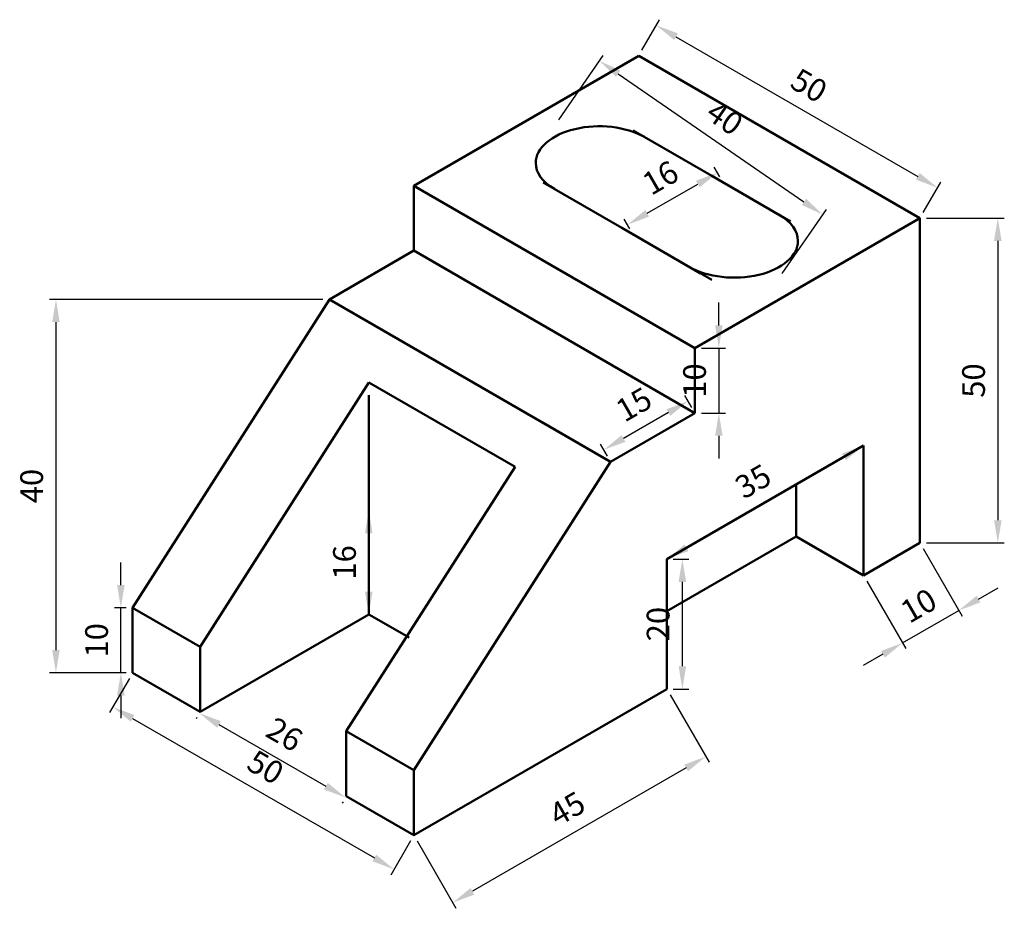
# Model space of a CAD drawing. Units: millimetres. Extents: x 2816 to 2967, y 623 to 760.
import ezdxf

# ---------------------------------------------------------------- set-up
doc = ezdxf.new("R2010")
doc.units = ezdxf.units.MM
doc.layers.add('M-DIMS', color=3, linetype='Continuous', lineweight=25)
doc.layers.add('M-OUTL', color=7, linetype='Continuous', lineweight=50)
doc.styles.get("Standard").update_dxf_attribs({"font": 'arial.ttf'})
doc.dimstyles.new('AM_ISO$0', dxfattribs={"dimtxt": 3.5, "dimasz": 3.5, "dimexe": 1, "dimexo": 1, "dimgap": 1.5, "dimtad": 1, "dimdsep": 46, "dimtxsty": 'Standard', "dimcen": 0, "dimclrd": 256, "dimclre": 256, "dimclrt": 2, "dimadec": 0, "dimazin": 2, "dimtp": 0.1, "dimtm": 0.1, "dimtfac": 0.71, "dimtdec": 3, "dimtmove": 0, "dimatfit": 3, "dimfxl": 1, "dimlwd": -1, "dimlwe": -1, "dimarcsym": 1})

# ---------------------------------------------------------------- blocks, each defined once
blk = doc.blocks.new('*D3')
at = {"layer": 'Defpoints', "color": 0, "transparency": 16777216}
for p in [(2954.44, 729.55), (2954.44, 679.55), (2966.44, 679.55)]:
    blk.add_point(p, dxfattribs=at)
at = {"layer": 'M-DIMS', "color": 0, "linetype": 'ByBlock', "transparency": 16777216}
for p, q in [((2955.44, 729.55), (2967.44, 729.55)), ((2966.44, 726.05), (2966.44, 683.05)), ((2955.44, 679.55), (2967.44, 679.55))]:
    blk.add_line(p, q, dxfattribs=at)
at = {"layer": 'M-DIMS', "color": 0, "transparency": 16777216}
for points in [[(2965.86, 726.05), (2967.03, 726.05), (2966.44, 729.55)], [(2965.86, 683.05), (2967.03, 683.05), (2966.44, 679.55)]]:
    blk.add_solid(points, dxfattribs=at)
at = {"layer": 'M-DIMS', "color": 0, "transparency": 16777216, "insert": (2963.16, 704.55), "char_height": 3.5, "attachment_point": 5, "rotation": 90}
blk.add_mtext('50', dxfattribs=at)
blk = doc.blocks.new('*D4')
at = {"layer": 'Defpoints', "color": 0, "transparency": 16777216}
for p in [(2911.14, 754.55), (2957.15, 734.24), (2954.44, 729.55)]:
    blk.add_point(p, dxfattribs=at)
at = {"layer": 'M-DIMS', "color": 0, "linetype": 'ByBlock', "transparency": 16777216}
for p, q in [((2911.64, 755.42), (2914.35, 760.11)), ((2916.88, 757.49), (2954.12, 735.99)), ((2954.94, 730.42), (2957.65, 735.11))]:
    blk.add_line(p, q, dxfattribs=at)
at = {"layer": 'M-DIMS', "color": 0, "transparency": 16777216}
for points in [[(2917.17, 758), (2916.59, 756.99), (2913.85, 759.24)], [(2954.41, 736.5), (2953.83, 735.49), (2957.15, 734.24)]]:
    blk.add_solid(points, dxfattribs=at)
at = {"layer": 'M-DIMS', "color": 0, "transparency": 16777216, "insert": (2937.14, 749.59), "char_height": 3.5, "attachment_point": 5, "rotation": 330}
blk.add_mtext('50', dxfattribs=at)
blk = doc.blocks.new('*D5')
at = {"layer": 'Defpoints', "color": 0, "transparency": 16777216}
for p in [(2898.29, 743.89), (2939.47, 730.09), (2932.67, 720.21)]:
    blk.add_point(p, dxfattribs=at)
at = {"layer": 'M-DIMS', "color": 0, "linetype": 'ByBlock', "transparency": 16777216}
for p, q in [((2898.85, 744.71), (2905.66, 754.6)), ((2907.97, 751.79), (2936.59, 732.07)), ((2933.23, 721.03), (2940.04, 730.91))]:
    blk.add_line(p, q, dxfattribs=at)
at = {"layer": 'M-DIMS', "color": 0, "transparency": 16777216}
for points in [[(2908.31, 752.27), (2907.64, 751.31), (2905.09, 753.77)], [(2936.92, 732.55), (2936.26, 731.59), (2939.47, 730.09)]]:
    blk.add_solid(points, dxfattribs=at)
at = {"layer": 'M-DIMS', "color": 0, "transparency": 16777216, "insert": (2924.15, 744.64), "char_height": 3.5, "attachment_point": 5, "rotation": 325.4399}
blk.add_mtext('40', dxfattribs=at)
blk = doc.blocks.new('*D6')
at = {"layer": 'Defpoints', "color": 0, "transparency": 16777216}
for p in [(2923.27, 736.56), (2924.14, 735.06), (2910.27, 727.05)]:
    blk.add_point(p, dxfattribs=at)
at = {"layer": 'M-DIMS', "color": 0, "linetype": 'ByBlock', "transparency": 16777216}
for p, q in [((2923.64, 735.93), (2922.77, 737.42)), ((2912.44, 730.3), (2920.24, 734.81)), ((2909.77, 727.92), (2908.91, 729.42))]:
    blk.add_line(p, q, dxfattribs=at)
at = {"layer": 'M-DIMS', "color": 0, "transparency": 16777216}
for points in [[(2919.95, 735.31), (2920.53, 734.3), (2923.27, 736.56)], [(2912.15, 730.8), (2912.73, 729.79), (2909.41, 728.55)]]:
    blk.add_solid(points, dxfattribs=at)
at = {"layer": 'M-DIMS', "color": 0, "transparency": 16777216, "insert": (2914.7, 735.4), "char_height": 3.5, "attachment_point": 5, "rotation": 30}
blk.add_mtext('16', dxfattribs=at)
blk = doc.blocks.new('*D7')
at = {"layer": 'Defpoints', "color": 0, "transparency": 16777216}
for p in [(2919.8, 709.55), (2919.8, 699.55), (2923.48, 699.55)]:
    blk.add_point(p, dxfattribs=at)
at = {"layer": 'M-DIMS', "color": 0, "linetype": 'ByBlock', "transparency": 16777216}
for p, q in [((2923.48, 713.05), (2923.48, 716.55)), ((2920.8, 709.55), (2924.48, 709.55)), ((2923.48, 709.55), (2923.48, 699.55)), ((2920.8, 699.55), (2924.48, 699.55)), ((2923.48, 696.05), (2923.48, 692.55))]:
    blk.add_line(p, q, dxfattribs=at)
at = {"layer": 'M-DIMS', "color": 0, "transparency": 16777216}
for points in [[(2922.9, 713.05), (2924.06, 713.05), (2923.48, 709.55)], [(2922.9, 696.05), (2924.06, 696.05), (2923.48, 699.55)]]:
    blk.add_solid(points, dxfattribs=at)
at = {"layer": 'M-DIMS', "color": 0, "transparency": 16777216, "insert": (2920.19, 704.55), "char_height": 3.5, "attachment_point": 5, "rotation": 90}
blk.add_mtext('10', dxfattribs=at)
blk = doc.blocks.new('*D8')
at = {"layer": 'Defpoints', "color": 0, "transparency": 16777216}
for p in [(2919.8, 699.55), (2905.75, 693.88), (2906.81, 692.05)]:
    blk.add_point(p, dxfattribs=at)
at = {"layer": 'M-DIMS', "color": 0, "linetype": 'ByBlock', "transparency": 16777216}
for p, q in [((2919.3, 700.42), (2918.25, 702.25)), ((2915.71, 699.63), (2908.79, 695.63)), ((2906.31, 692.92), (2905.25, 694.75))]:
    blk.add_line(p, q, dxfattribs=at)
at = {"layer": 'M-DIMS', "color": 0, "transparency": 16777216}
for points in [[(2915.42, 700.13), (2916.01, 699.12), (2918.75, 701.38)], [(2908.49, 696.13), (2909.08, 695.12), (2905.75, 693.88)]]:
    blk.add_solid(points, dxfattribs=at)
at = {"layer": 'M-DIMS', "color": 0, "transparency": 16777216, "insert": (2910.61, 700.48), "char_height": 3.5, "attachment_point": 5, "rotation": 30}
blk.add_mtext('15', dxfattribs=at)
blk = doc.blocks.new('*D9')
at = {"layer": 'Defpoints', "color": 0, "transparency": 16777216}
for p in [(2869.57, 684.55), (2869.57, 684.55), (2869.57, 668.55)]:
    blk.add_point(p, dxfattribs=at)
at = {"layer": 'M-DIMS', "color": 0, "linetype": 'ByBlock', "transparency": 16777216}
blk.add_line((2869.57, 672.05), (2869.57, 681.05), dxfattribs=at)
at = {"layer": 'M-DIMS', "color": 0, "transparency": 16777216}
for points in [[(2868.99, 681.05), (2870.15, 681.05), (2869.57, 684.55)], [(2868.99, 672.05), (2870.15, 672.05), (2869.57, 668.55)]]:
    blk.add_solid(points, dxfattribs=at)
at = {"layer": 'M-DIMS', "color": 0, "transparency": 16777216, "insert": (2866.28, 676.55), "char_height": 3.5, "attachment_point": 5, "rotation": 90}
blk.add_mtext('16', dxfattribs=at)
blk = doc.blocks.new('*D10')
at = {"layer": 'Defpoints', "color": 0, "transparency": 16777216}
for p in [(2843.59, 653.55), (2865.99, 640.35), (2866.11, 640.55)]:
    blk.add_point(p, dxfattribs=at)
at = {"layer": 'M-DIMS', "color": 0, "linetype": 'ByBlock', "transparency": 16777216}
for p, q in [((2843.09, 652.68), (2842.97, 652.48)), ((2846.5, 651.6), (2862.96, 642.1)), ((2865.61, 639.68), (2865.49, 639.48))]:
    blk.add_line(p, q, dxfattribs=at)
at = {"layer": 'M-DIMS', "color": 0, "transparency": 16777216}
for points in [[(2846.8, 652.1), (2846.21, 651.09), (2843.47, 653.35)], [(2863.25, 642.6), (2862.67, 641.59), (2865.99, 640.35)]]:
    blk.add_solid(points, dxfattribs=at)
at = {"layer": 'M-DIMS', "color": 0, "transparency": 16777216, "insert": (2856.37, 649.69), "char_height": 3.5, "attachment_point": 5, "rotation": 330}
blk.add_mtext('26', dxfattribs=at)
blk = doc.blocks.new('*D11')
at = {"layer": 'Defpoints', "color": 0, "transparency": 16777216}
for p in [(2833.2, 659.55), (2876.5, 634.55), (2873.46, 629.29)]:
    blk.add_point(p, dxfattribs=at)
at = {"layer": 'M-DIMS', "color": 0, "linetype": 'ByBlock', "transparency": 16777216}
for p, q in [((2832.7, 658.68), (2829.66, 653.42)), ((2833.19, 652.54), (2870.43, 631.04)), ((2876, 633.68), (2872.96, 628.42))]:
    blk.add_line(p, q, dxfattribs=at)
at = {"layer": 'M-DIMS', "color": 0, "transparency": 16777216}
for points in [[(2833.48, 653.04), (2832.9, 652.03), (2830.16, 654.29)], [(2870.72, 631.54), (2870.14, 630.53), (2873.46, 629.29)]]:
    blk.add_solid(points, dxfattribs=at)
at = {"layer": 'M-DIMS', "color": 0, "transparency": 16777216, "insert": (2853.45, 644.63), "char_height": 3.5, "attachment_point": 5, "rotation": 330}
blk.add_mtext('50', dxfattribs=at)
blk = doc.blocks.new('*D12')
at = {"layer": 'Defpoints', "color": 0, "transparency": 16777216}
for p in [(2915.47, 657.05), (2876.5, 634.55), (2882.5, 624.16)]:
    blk.add_point(p, dxfattribs=at)
at = {"layer": 'M-DIMS', "color": 0, "linetype": 'ByBlock', "transparency": 16777216}
for p, q in [((2915.97, 656.18), (2921.97, 645.79)), ((2918.44, 644.91), (2885.53, 625.91)), ((2877, 633.68), (2883, 623.29))]:
    blk.add_line(p, q, dxfattribs=at)
at = {"layer": 'M-DIMS', "color": 0, "transparency": 16777216}
for points in [[(2918.15, 645.41), (2918.73, 644.4), (2921.47, 646.66)], [(2885.24, 626.41), (2885.82, 625.4), (2882.5, 624.16)]]:
    blk.add_solid(points, dxfattribs=at)
at = {"layer": 'M-DIMS', "color": 0, "transparency": 16777216, "insert": (2900.35, 638.25), "char_height": 3.5, "attachment_point": 5, "rotation": 30}
blk.add_mtext('45', dxfattribs=at)
blk = doc.blocks.new('*D13')
at = {"layer": 'Defpoints', "color": 0, "transparency": 16777216}
for p in [(2915.47, 677.05), (2917.86, 677.05), (2915.47, 657.05)]:
    blk.add_point(p, dxfattribs=at)
at = {"layer": 'M-DIMS', "color": 0, "linetype": 'ByBlock', "transparency": 16777216}
for p, q in [((2916.47, 677.05), (2918.86, 677.05)), ((2917.86, 660.55), (2917.86, 673.55)), ((2916.47, 657.05), (2918.86, 657.05))]:
    blk.add_line(p, q, dxfattribs=at)
at = {"layer": 'M-DIMS', "color": 0, "transparency": 16777216}
for points in [[(2917.28, 673.55), (2918.45, 673.55), (2917.86, 677.05)], [(2917.28, 660.55), (2918.45, 660.55), (2917.86, 657.05)]]:
    blk.add_solid(points, dxfattribs=at)
at = {"layer": 'M-DIMS', "color": 0, "transparency": 16777216, "insert": (2914.58, 667.05), "char_height": 3.5, "attachment_point": 5, "rotation": 90}
blk.add_mtext('20', dxfattribs=at)
blk = doc.blocks.new('*D14')
at = {"layer": 'Defpoints', "color": 0, "transparency": 16777216}
for p in [(2945.78, 694.55), (2945.78, 694.55), (2915.47, 677.05)]:
    blk.add_point(p, dxfattribs=at)
at = {"layer": 'M-DIMS', "color": 0, "linetype": 'ByBlock', "transparency": 16777216}
blk.add_line((2918.5, 678.8), (2942.75, 692.8), dxfattribs=at)
at = {"layer": 'M-DIMS', "color": 0, "transparency": 16777216}
for points in [[(2942.46, 693.31), (2943.04, 692.3), (2945.78, 694.55)], [(2918.21, 679.31), (2918.79, 678.3), (2915.47, 677.05)]]:
    blk.add_solid(points, dxfattribs=at)
at = {"layer": 'M-DIMS', "color": 0, "transparency": 16777216, "insert": (2928.98, 688.65), "char_height": 3.5, "attachment_point": 5, "rotation": 30}
blk.add_mtext('35', dxfattribs=at)
blk = doc.blocks.new('*D15')
at = {"layer": 'Defpoints', "color": 0, "transparency": 16777216}
for p in [(2954.44, 679.55), (2945.78, 674.55), (2960.44, 669.16)]:
    blk.add_point(p, dxfattribs=at)
at = {"layer": 'M-DIMS', "color": 0, "linetype": 'ByBlock', "transparency": 16777216}
for p, q in [((2954.94, 678.68), (2960.94, 668.29)), ((2946.28, 673.68), (2952.28, 663.29)), ((2963.47, 670.91), (2966.5, 672.66)), ((2951.78, 664.16), (2960.44, 669.16)), ((2948.75, 662.41), (2945.72, 660.66))]:
    blk.add_line(p, q, dxfattribs=at)
at = {"layer": 'M-DIMS', "color": 0, "transparency": 16777216}
for points in [[(2963.18, 671.41), (2963.76, 670.4), (2960.44, 669.16)], [(2948.46, 662.91), (2949.04, 661.9), (2951.78, 664.16)]]:
    blk.add_solid(points, dxfattribs=at)
at = {"layer": 'M-DIMS', "color": 0, "transparency": 16777216, "insert": (2954.47, 669.51), "char_height": 3.5, "attachment_point": 5, "rotation": 30}
blk.add_mtext('10', dxfattribs=at)
blk = doc.blocks.new('*D16')
at = {"layer": 'Defpoints', "color": 0, "transparency": 16777216}
for p in [(2831.39, 669.55), (2833.2, 669.55), (2833.2, 659.55)]:
    blk.add_point(p, dxfattribs=at)
at = {"layer": 'M-DIMS', "color": 0, "linetype": 'ByBlock', "transparency": 16777216}
for p, q in [((2831.39, 673.05), (2831.39, 676.55)), ((2832.2, 669.55), (2830.39, 669.55)), ((2831.39, 659.55), (2831.39, 669.55)), ((2832.2, 659.55), (2830.39, 659.55)), ((2831.39, 656.05), (2831.39, 652.55))]:
    blk.add_line(p, q, dxfattribs=at)
at = {"layer": 'M-DIMS', "color": 0, "transparency": 16777216}
for points in [[(2830.81, 673.05), (2831.97, 673.05), (2831.39, 669.55)], [(2830.81, 656.05), (2831.97, 656.05), (2831.39, 659.55)]]:
    blk.add_solid(points, dxfattribs=at)
at = {"layer": 'M-DIMS', "color": 0, "transparency": 16777216, "insert": (2828.1, 664.55), "char_height": 3.5, "attachment_point": 5, "rotation": 90}
blk.add_mtext('10', dxfattribs=at)
blk = doc.blocks.new('*D17')
at = {"layer": 'Defpoints', "color": 0, "transparency": 16777216}
for p in [(2863.51, 717.05), (2821.39, 659.55), (2833.2, 659.55)]:
    blk.add_point(p, dxfattribs=at)
at = {"layer": 'M-DIMS', "color": 0, "linetype": 'ByBlock', "transparency": 16777216}
for p, q in [((2862.51, 717.05), (2820.39, 717.05)), ((2821.39, 713.55), (2821.39, 663.05)), ((2832.2, 659.55), (2820.39, 659.55))]:
    blk.add_line(p, q, dxfattribs=at)
at = {"layer": 'M-DIMS', "color": 0, "transparency": 16777216}
for points in [[(2820.81, 713.55), (2821.97, 713.55), (2821.39, 717.05)], [(2820.81, 663.05), (2821.97, 663.05), (2821.39, 659.55)]]:
    blk.add_solid(points, dxfattribs=at)
at = {"layer": 'M-DIMS', "color": 0, "transparency": 16777216, "insert": (2818.1, 688.3), "char_height": 3.5, "attachment_point": 5, "rotation": 90}
blk.add_mtext('40', dxfattribs=at)

msp = doc.modelspace()

# ---------------------------------------------------------------- linework, layer by layer
at = {"layer": 'M-OUTL'}
for p, q in [((2876.5, 734.551), (2911.141, 754.551)), ((2911.141, 754.551), (2954.442, 729.551)), ((2922.399, 736.051), (2910.28, 743.048)), ((2934.529, 729.048), (2922.399, 736.051)), ((2919.801, 709.551), (2876.5, 734.551)), ((2876.5, 734.551), (2876.5, 724.551)), ((2896.424, 735.048), (2908.543, 728.051)), ((2924.136, 735.06), (2924.126, 735.054)), ((2954.442, 729.551), (2919.801, 709.551)), ((2954.442, 679.551), (2954.442, 729.551)), ((2908.543, 728.051), (2920.672, 721.048)), ((2910.269, 727.054), (2922.399, 720.051)), ((2876.5, 724.551), (2863.509, 717.051)), ((2919.801, 699.551), (2876.5, 724.551)), ((2833.198, 669.551), (2863.509, 717.051)), ((2863.509, 717.051), (2906.811, 692.051)), ((2919.801, 709.551), (2919.801, 699.551)), ((2869.572, 704.265), (2843.591, 663.551)), ((2892.088, 691.265), (2869.572, 704.265)), ((2869.572, 668.551), (2869.572, 702.315)), ((2919.801, 699.551), (2906.811, 692.051)), ((2906.811, 692.051), (2896.418, 698.051)), ((2915.471, 677.051), (2945.782, 694.551)), ((2945.782, 694.551), (2945.782, 674.551)), ((2876.5, 644.551), (2906.811, 692.051)), ((2892.088, 691.265), (2866.107, 650.551)), ((2935.389, 680.551), (2935.389, 688.551)), ((2869.572, 668.551), (2869.572, 684.551)), ((2915.471, 669.051), (2935.389, 680.551)), ((2945.782, 674.551), (2935.389, 680.551)), ((2945.782, 674.551), (2954.442, 679.551)), ((2915.471, 657.051), (2915.471, 677.051)), ((2843.591, 663.551), (2833.198, 669.551)), ((2833.198, 669.551), (2833.198, 659.551)), ((2869.572, 668.551), (2843.591, 653.551)), ((2875.772, 664.971), (2869.572, 668.551)), ((2843.591, 653.551), (2843.591, 663.551)), ((2833.198, 659.551), (2843.591, 653.551)), ((2876.5, 634.551), (2915.471, 657.051)), ((2876.5, 644.551), (2866.107, 650.551)), ((2866.107, 650.551), (2866.107, 640.551)), ((2876.5, 634.551), (2876.5, 644.551)), ((2866.107, 640.551), (2876.5, 634.551))]:
    msp.add_line(p, q, dxfattribs=at)
for centre, start_param, end_param in [((2905.079, 738.051), 3.9269908, 6.2831853), ((2905.079, 738.051), 0, 0.7853982), ((2925.863, 726.051), 3.1415927, 3.9269908), ((2925.863, 726.051), 0.7853982, 3.1415927)]:
    msp.add_ellipse(centre, major_axis=(-9.798, 0), ratio=0.5773503, start_param=start_param, end_param=end_param, dxfattribs=at)

# ---------------------------------------------------------------- dimensions: what is measured, and where the dimension line sits
at = {"layer": 'M-DIMS'}
for p1, p2, distance, override, picture, middle in [((2911.141, 754.551), (2954.442, 729.551), 5.419, {"dimpost": '', "dimclrd": 0, "dimclre": 0, "dimclrt": 0}, '*D4', (2937.144, 749.591)), ((2954.442, 729.551), (2954.442, 679.551), 12, {"dimpost": '', "dimclrd": 0, "dimclre": 0, "dimclrt": 0}, '*D3', (2963.155, 704.551)), ((2919.801, 709.551), (2919.801, 699.551), 3.679, {"dimclrd": 0, "dimclre": 0, "dimclrt": 0}, '*D7', (2920.193, 704.551)), ((2919.801, 699.551), (2906.811, 692.051), -2.112, {"dimclrd": 0, "dimclre": 0, "dimclrt": 0}, '*D8', (2910.606, 700.476)), ((2915.471, 677.051), (2945.782, 694.551), 0, {"dimclrd": 0, "dimclre": 0, "dimclrt": 0}, '*D14', (2928.982, 688.649)), ((2869.572, 668.551), (2869.572, 684.551), 0, {"dimclrd": 0, "dimclre": 0, "dimclrt": 0}, '*D9', (2866.285, 676.551)), ((2945.782, 674.551), (2954.442, 679.551), -12, {"dimclrd": 0, "dimclre": 0, "dimclrt": 0}, '*D15', (2954.468, 669.505)), ((2833.198, 659.551), (2833.198, 669.551), 1.807, {"dimclrd": 0, "dimclre": 0, "dimclrt": 0}, '*D16', (2828.105, 664.551)), ((2915.471, 657.051), (2915.471, 677.051), -2.393, {"dimclrd": 0, "dimclre": 0, "dimclrt": 0}, '*D13', (2914.577, 667.051)), ((2833.198, 659.551), (2876.5, 634.551), -6.078, {"dimclrd": 0, "dimclre": 0, "dimclrt": 0}, '*D11', (2853.454, 644.634)), ((2915.471, 657.051), (2876.5, 634.551), 12, {"dimclrd": 0, "dimclre": 0, "dimclrt": 0}, '*D12', (2900.345, 638.249)), ((2843.591, 653.551), (2866.107, 640.551), -0.235, {"dimclrd": 0, "dimclre": 0, "dimclrt": 0}, '*D10', (2856.375, 649.694))]:
    dim = msp.add_aligned_dim(p1=p1, p2=p2, distance=distance, dimstyle='AM_ISO$0', override=override, dxfattribs=at)
    dim.commit()
    dim.dimension.update_dxf_attribs({"geometry": picture, "text_midpoint": middle})
for p1, p2, distance, text, picture, middle in [((2898.285, 743.89), (2932.667, 720.206), 12, '40', '*D5', (2924.148, 744.637)), ((2910.269, 727.054), (2924.136, 735.06), 1.727, '16', '*D6', (2914.696, 735.399))]:
    dim = msp.add_aligned_dim(p1=p1, p2=p2, distance=distance, text=text, dimstyle='AM_ISO$0', override={"dimpost": '', "dimclrd": 0, "dimclre": 0, "dimclrt": 0}, dxfattribs=at)
    dim.commit()
    dim.dimension.update_dxf_attribs({"geometry": picture, "text_midpoint": middle})
dim = msp.add_linear_dim(base=(2821.392, 659.551), p1=(2863.509, 717.051), p2=(2833.198, 659.551), angle=90, text='40', dimstyle='AM_ISO$0', override={"dimpost": '', "dimclrd": 0, "dimclre": 0, "dimclrt": 0}, dxfattribs=at)
dim.commit()
dim.dimension.update_dxf_attribs({"geometry": '*D17', "text_midpoint": (2818.105, 688.301)})

doc.saveas('drawing.dxf')
